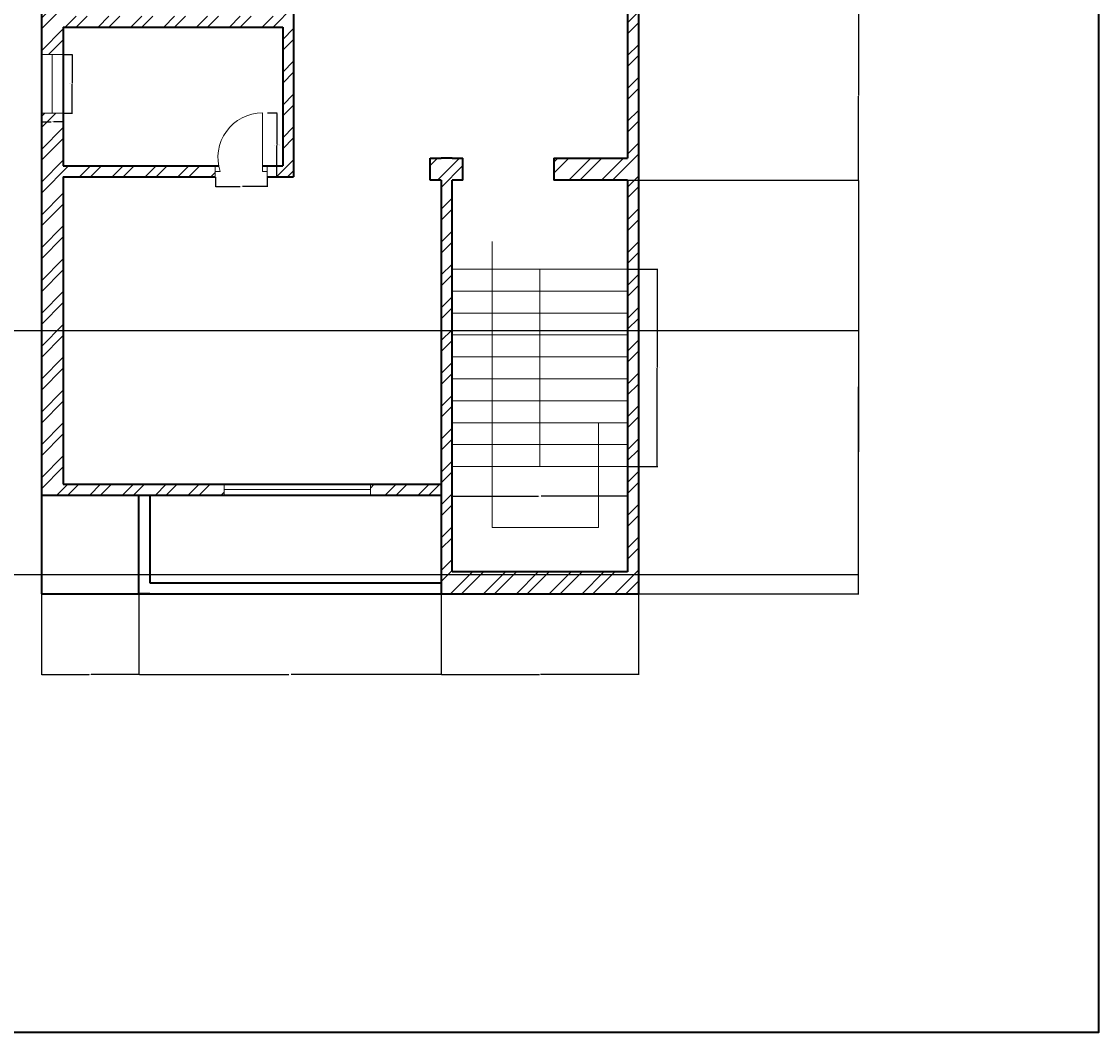
# Model space of a CAD drawing. Units: inches. Extents: x 1850 to 3445, y 1558 to 2756.
# Tile 11 of 13: x 3003 to 3445, y 1558 to 1972. Entities that reach past the tile are written whole.
import ezdxf

# ---------------------------------------------------------------- set-up
doc = ezdxf.new("R2010")
doc.units = ezdxf.units.IN
for name, color, linetype, lineweight in [('A-ANNO-DIMS', 2, 'Continuous', 18), ('A-ANNO-TTLB', 7, 'Continuous', 35), ('A-DOOR', 3, 'Continuous', 18), ('A-FLOR-STRS', 7, 'Continuous', 18), ('A-GLAZ', 4, 'Continuous', 18), ('A-WALL', 7, 'Continuous', 35), ('A-WALL-PATT', 252, 'Continuous', 13)]:
    doc.layers.add(name, color=color, linetype=linetype, lineweight=lineweight)
doc.styles.get("Standard").update_dxf_attribs({"font": 'arial.ttf'})
doc.dimstyles.get("Standard").update_dxf_attribs({"dimtxt": 0.18, "dimasz": 0.18, "dimexe": 0.18, "dimexo": 0.0625, "dimgap": 0.09, "dimtad": 0, "dimtih": 1, "dimtoh": 1, "dimdec": 4, "dimzin": 0, "dimdsep": 46, "dimtxsty": 'Standard', "dimcen": 0.09, "dimadec": 0, "dimazin": 0, "dimtfac": 1, "dimtdec": 4, "dimtofl": 0, "dimtmove": 0, "dimatfit": 3, "dimfxl": 1, "dimtolj": 1, "dimtzin": 0, "dimarcsym": 0})
pattern_1 = [(45, (660.551, 0), (-6.735192, 6.735192), []), (45, (665.041, 0), (-6.735192, 6.735192), [])]

# ---------------------------------------------------------------- blocks, each defined once
blk = doc.blocks.new('WIN-24-W9')
for p, q in [((9, 24), (0, 24)), ((0, 24), (4.5, 24)), ((4.5, 24), (4.5, 0)), ((9, 0), (0, 0)), ((4.5, 0), (9, 0))]:
    blk.add_line(p, q)
blk = doc.blocks.new('WIN-60-W4_5')
for p, q in [((0, 60), (4.5, 60)), ((4.5, 60), (2.25, 60)), ((2.25, 60), (2.25, 0)), ((2.25, 0), (0, 0)), ((0, 0), (4.5, 0))]:
    blk.add_line(p, q)
blk = doc.blocks.new('DOOR-BATH-LOWER-HALL')
for p, q in [((19.31, 2.25), (19.31, 26.25)), ((0, 4.5), (0, 0)), ((21.31, 4.5), (21.31, 0)), ((0, 0), (0, 2.25)), ((0, 2.25), (2, 2.25)), ((21.31, 2.25), (19.31, 2.25)), ((21.31, 0), (21.31, 2.25))]:
    blk.add_line(p, q)
blk.add_arc((19.31, 8.01), 18.24, 90, 198.4026)
blk = doc.blocks.new('STAIR-UPPER-FLIGHT')
for p, q in [((72, 81), (0, 81)), ((36, 0), (36, 81)), ((72, 72), (0, 72)), ((72, 63), (0, 63)), ((72, 54), (0, 54)), ((72, 45), (0, 45)), ((72, 36), (0, 36)), ((72, 27), (0, 27)), ((72, 18), (0, 18)), ((72, 9), (0, 9)), ((0, 0), (72, 0)), ((72, 0), (36, 0))]:
    blk.add_line(p, q)
blk = doc.blocks.new('*D40')
at = {"layer": 'A-ANNO-DIMS', "color": 0, "lineweight": -2, "transparency": 16777216}
for p, q in [((3020.67, 1958.91), (3024.39, 1958.91)), ((3024.21, 1958.73), (3024.21, 1947.1)), ((3024.21, 1935.09), (3024.21, 1946.73)), ((3020.67, 1934.91), (3024.39, 1934.91))]:
    blk.add_line(p, q, dxfattribs=at)
at = {"layer": 'A-ANNO-DIMS', "color": 0, "transparency": 16777216}
for points in [[(3024.18, 1958.73), (3024.24, 1958.73), (3024.21, 1958.91)], [(3024.18, 1935.09), (3024.24, 1935.09), (3024.21, 1934.91)]]:
    blk.add_solid(points, dxfattribs=at)
at = {"layer": 'Defpoints', "color": 0, "transparency": 16777216}
for p in [(3020.61, 1958.91), (3024.21, 1958.91), (3020.61, 1934.91)]:
    blk.add_point(p, dxfattribs=at)
at = {"layer": 'A-ANNO-DIMS', "color": 0, "transparency": 16777216, "insert": (3024.21, 1946.91), "char_height": 0.18, "attachment_point": 5}
blk.add_mtext('\\A1;WINDOW 24 TYP.', dxfattribs=at)
blk = doc.blocks.new('*D41')
at = {"layer": 'A-ANNO-DIMS', "color": 0, "lineweight": -2, "transparency": 16777216}
for p, q in [((3011.61, 1934.85), (3011.61, 1931.13)), ((3011.79, 1931.31), (3015.65, 1931.31)), ((3020.43, 1931.31), (3016.56, 1931.31)), ((3020.61, 1934.85), (3020.61, 1931.13))]:
    blk.add_line(p, q, dxfattribs=at)
at = {"layer": 'A-ANNO-DIMS', "color": 0, "transparency": 16777216}
for points in [[(3011.79, 1931.34), (3011.79, 1931.28), (3011.61, 1931.31)], [(3020.43, 1931.34), (3020.43, 1931.28), (3020.61, 1931.31)]]:
    blk.add_solid(points, dxfattribs=at)
at = {"layer": 'Defpoints', "color": 0, "transparency": 16777216}
for p in [(3011.61, 1934.91), (3020.61, 1934.91), (3020.61, 1931.31)]:
    blk.add_point(p, dxfattribs=at)
at = {"layer": 'A-ANNO-DIMS', "color": 0, "transparency": 16777216, "insert": (3016.11, 1931.31), "char_height": 0.18, "attachment_point": 5}
blk.add_mtext('\\A1;9 TYP.', dxfattribs=at)
blk = doc.blocks.new('*D66')
at = {"layer": 'A-ANNO-DIMS', "color": 0, "lineweight": -2, "transparency": 16777216}
for p, q in [((3104.35, 1934.93), (3108.4, 1934.93)), ((3108.22, 1934.75), (3108.22, 1921.99)), ((3108.22, 1908.86), (3108.22, 1921.63)), ((3104.35, 1908.68), (3108.4, 1908.68))]:
    blk.add_line(p, q, dxfattribs=at)
at = {"layer": 'A-ANNO-DIMS', "color": 0, "transparency": 16777216}
for points in [[(3108.19, 1934.75), (3108.25, 1934.75), (3108.22, 1934.93)], [(3108.19, 1908.86), (3108.25, 1908.86), (3108.22, 1908.68)]]:
    blk.add_solid(points, dxfattribs=at)
at = {"layer": 'Defpoints', "color": 0, "transparency": 16777216}
for p in [(3104.28, 1934.93), (3108.22, 1934.93), (3104.28, 1908.68)]:
    blk.add_point(p, dxfattribs=at)
at = {"layer": 'A-ANNO-DIMS', "color": 0, "transparency": 16777216, "insert": (3108.22, 1921.81), "char_height": 0.18, "attachment_point": 5}
blk.add_mtext('\\A1;BATH DOOR 26 TYP.', dxfattribs=at)
blk = doc.blocks.new('*D67')
at = {"layer": 'A-ANNO-DIMS', "color": 0, "lineweight": -2, "transparency": 16777216}
for p, q in [((3082.98, 1908.62), (3082.98, 1904.57)), ((3104.28, 1908.62), (3104.28, 1904.57)), ((3083.16, 1904.75), (3093.1, 1904.75)), ((3104.1, 1904.75), (3094.16, 1904.75))]:
    blk.add_line(p, q, dxfattribs=at)
at = {"layer": 'A-ANNO-DIMS', "color": 0, "transparency": 16777216}
for points in [[(3083.16, 1904.78), (3083.16, 1904.72), (3082.98, 1904.75)], [(3104.1, 1904.78), (3104.1, 1904.72), (3104.28, 1904.75)]]:
    blk.add_solid(points, dxfattribs=at)
at = {"layer": 'Defpoints', "color": 0, "transparency": 16777216}
for p in [(3082.98, 1908.68), (3104.28, 1908.68), (3104.28, 1904.75)]:
    blk.add_point(p, dxfattribs=at)
at = {"layer": 'A-ANNO-DIMS', "color": 0, "transparency": 16777216, "insert": (3093.63, 1904.75), "char_height": 0.18, "attachment_point": 5}
blk.add_mtext('\\A1;21 TYP.', dxfattribs=at)
blk = doc.blocks.new('*D70')
at = {"layer": 'A-ANNO-DIMS', "color": 0, "lineweight": -2, "transparency": 16777216}
for p, q in [((3252.17, 1870.88), (3264.44, 1870.88)), ((3264.26, 1870.7), (3264.26, 1830.56)), ((3264.26, 1790.06), (3264.26, 1830.2)), ((3252.17, 1789.88), (3264.44, 1789.88))]:
    blk.add_line(p, q, dxfattribs=at)
at = {"layer": 'A-ANNO-DIMS', "color": 0, "transparency": 16777216}
for points in [[(3264.23, 1870.7), (3264.29, 1870.7), (3264.26, 1870.88)], [(3264.23, 1790.06), (3264.29, 1790.06), (3264.26, 1789.88)]]:
    blk.add_solid(points, dxfattribs=at)
at = {"layer": 'Defpoints', "color": 0, "transparency": 16777216}
for p in [(3252.11, 1870.88), (3264.26, 1870.88), (3252.11, 1789.88)]:
    blk.add_point(p, dxfattribs=at)
at = {"layer": 'A-ANNO-DIMS', "color": 0, "transparency": 16777216, "insert": (3264.26, 1830.38), "char_height": 0.18, "attachment_point": 5}
blk.add_mtext('\\A1;STAIR FLIGHT 81 TYP.', dxfattribs=at)
blk = doc.blocks.new('*D71')
at = {"layer": 'A-ANNO-DIMS', "color": 0, "lineweight": -2, "transparency": 16777216}
for p, q in [((3180.11, 1789.82), (3180.11, 1777.55)), ((3252.11, 1789.82), (3252.11, 1777.55)), ((3180.29, 1777.73), (3215.58, 1777.73)), ((3251.93, 1777.73), (3216.63, 1777.73))]:
    blk.add_line(p, q, dxfattribs=at)
at = {"layer": 'A-ANNO-DIMS', "color": 0, "transparency": 16777216}
for points in [[(3180.29, 1777.76), (3180.29, 1777.7), (3180.11, 1777.73)], [(3251.93, 1777.76), (3251.93, 1777.7), (3252.11, 1777.73)]]:
    blk.add_solid(points, dxfattribs=at)
at = {"layer": 'Defpoints', "color": 0, "transparency": 16777216}
for p in [(3180.11, 1789.88), (3252.11, 1789.88), (3252.11, 1777.73)]:
    blk.add_point(p, dxfattribs=at)
at = {"layer": 'A-ANNO-DIMS', "color": 0, "transparency": 16777216, "insert": (3216.11, 1777.73), "char_height": 0.18, "attachment_point": 5}
blk.add_mtext('\\A1;72 TYP.', dxfattribs=at)
blk = doc.blocks.new('*D94')
at = {"layer": 'A-ANNO-DIMS', "color": 0, "lineweight": -2, "transparency": 16777216}
for p, q in [((3011.61, 1737.62), (3011.61, 1704.45)), ((3051.65, 1737.62), (3051.65, 1704.45)), ((3011.79, 1704.63), (3031.16, 1704.63)), ((3051.47, 1704.63), (3032.1, 1704.63))]:
    blk.add_line(p, q, dxfattribs=at)
at = {"layer": 'A-ANNO-DIMS', "color": 0, "transparency": 16777216}
for points in [[(3011.79, 1704.66), (3011.79, 1704.6), (3011.61, 1704.63)], [(3051.47, 1704.66), (3051.47, 1704.6), (3051.65, 1704.63)]]:
    blk.add_solid(points, dxfattribs=at)
at = {"layer": 'Defpoints', "color": 0, "transparency": 16777216}
for p in [(3011.61, 1737.68), (3051.65, 1737.68), (3051.65, 1704.63)]:
    blk.add_point(p, dxfattribs=at)
at = {"layer": 'A-ANNO-DIMS', "color": 0, "transparency": 16777216, "insert": (3031.63, 1704.63), "char_height": 0.18, "attachment_point": 5}
blk.add_mtext('\\A1;40.046', dxfattribs=at)
blk = doc.blocks.new('*D95')
at = {"layer": 'A-ANNO-DIMS', "color": 0, "lineweight": -2, "transparency": 16777216}
for p, q in [((3051.65, 1737.62), (3051.65, 1704.45)), ((3175.61, 1737.62), (3175.61, 1704.45)), ((3051.83, 1704.63), (3113.17, 1704.63)), ((3175.43, 1704.63), (3114.08, 1704.63))]:
    blk.add_line(p, q, dxfattribs=at)
at = {"layer": 'A-ANNO-DIMS', "color": 0, "transparency": 16777216}
for points in [[(3051.83, 1704.66), (3051.83, 1704.6), (3051.65, 1704.63)], [(3175.43, 1704.66), (3175.43, 1704.6), (3175.61, 1704.63)]]:
    blk.add_solid(points, dxfattribs=at)
at = {"layer": 'Defpoints', "color": 0, "transparency": 16777216}
for p in [(3051.65, 1737.68), (3175.61, 1737.68), (3175.61, 1704.63)]:
    blk.add_point(p, dxfattribs=at)
at = {"layer": 'A-ANNO-DIMS', "color": 0, "transparency": 16777216, "insert": (3113.63, 1704.63), "char_height": 0.18, "attachment_point": 5}
blk.add_mtext('\\A1;123.95', dxfattribs=at)
blk = doc.blocks.new('*D96')
at = {"layer": 'A-ANNO-DIMS', "color": 0, "lineweight": -2, "transparency": 16777216}
for p, q in [((3175.61, 1737.62), (3175.61, 1704.45)), ((3256.61, 1737.62), (3256.61, 1704.45)), ((3175.79, 1704.63), (3215.9, 1704.63)), ((3256.43, 1704.63), (3216.31, 1704.63))]:
    blk.add_line(p, q, dxfattribs=at)
at = {"layer": 'A-ANNO-DIMS', "color": 0, "transparency": 16777216}
for points in [[(3175.79, 1704.66), (3175.79, 1704.6), (3175.61, 1704.63)], [(3256.43, 1704.66), (3256.43, 1704.6), (3256.61, 1704.63)]]:
    blk.add_solid(points, dxfattribs=at)
at = {"layer": 'Defpoints', "color": 0, "transparency": 16777216}
for p in [(3175.61, 1737.68), (3256.61, 1737.68), (3256.61, 1704.63)]:
    blk.add_point(p, dxfattribs=at)
at = {"layer": 'A-ANNO-DIMS', "color": 0, "transparency": 16777216, "insert": (3216.11, 1704.63), "char_height": 0.18, "attachment_point": 5}
blk.add_mtext('\\A1;81', dxfattribs=at)
blk = doc.blocks.new('*D102')
at = {"layer": 'A-ANNO-DIMS', "color": 0, "lineweight": -2, "transparency": 16777216}
for p, q in [((2941.38, 1845.68), (3346.97, 1845.68)), ((3346.79, 1845.5), (3346.79, 1795.87)), ((3346.79, 1745.86), (3346.79, 1795.5)), ((2945.88, 1745.68), (3346.97, 1745.68))]:
    blk.add_line(p, q, dxfattribs=at)
at = {"layer": 'A-ANNO-DIMS', "color": 0, "transparency": 16777216}
for points in [[(3346.76, 1845.5), (3346.82, 1845.5), (3346.79, 1845.68)], [(3346.76, 1745.86), (3346.82, 1745.86), (3346.79, 1745.68)]]:
    blk.add_solid(points, dxfattribs=at)
at = {"layer": 'Defpoints', "color": 0, "transparency": 16777216}
for p in [(2941.32, 1845.68), (3346.79, 1845.68), (2945.82, 1745.68)]:
    blk.add_point(p, dxfattribs=at)
at = {"layer": 'A-ANNO-DIMS', "color": 0, "transparency": 16777216, "insert": (3346.79, 1795.68), "char_height": 0.18, "attachment_point": 5}
blk.add_mtext('\\A1;100', dxfattribs=at)
blk = doc.blocks.new('*D103')
at = {"layer": 'A-ANNO-DIMS', "color": 0, "lineweight": -2, "transparency": 16777216}
for p, q in [((3252.17, 1907.39), (3346.97, 1907.39)), ((3346.79, 1907.21), (3346.79, 1822.72)), ((3346.79, 1737.86), (3346.79, 1822.36)), ((3256.67, 1737.68), (3346.97, 1737.68))]:
    blk.add_line(p, q, dxfattribs=at)
at = {"layer": 'A-ANNO-DIMS', "color": 0, "transparency": 16777216}
for points in [[(3346.76, 1907.21), (3346.82, 1907.21), (3346.79, 1907.39)], [(3346.76, 1737.86), (3346.82, 1737.86), (3346.79, 1737.68)]]:
    blk.add_solid(points, dxfattribs=at)
at = {"layer": 'Defpoints', "color": 0, "transparency": 16777216}
for p in [(3252.11, 1907.39), (3346.79, 1907.39), (3256.61, 1737.68)]:
    blk.add_point(p, dxfattribs=at)
at = {"layer": 'A-ANNO-DIMS', "color": 0, "transparency": 16777216, "insert": (3346.79, 1822.54), "char_height": 0.18, "attachment_point": 5}
blk.add_mtext('\\A1;169.7', dxfattribs=at)
blk = doc.blocks.new('*D104')
at = {"layer": 'A-ANNO-DIMS', "color": 0, "lineweight": -2, "transparency": 16777216}
for p, q in [((3256.67, 1976.5), (3346.97, 1976.5)), ((3346.79, 1976.32), (3346.79, 1942.13)), ((3346.79, 1907.57), (3346.79, 1941.76)), ((3252.17, 1907.39), (3346.97, 1907.39))]:
    blk.add_line(p, q, dxfattribs=at)
at = {"layer": 'A-ANNO-DIMS', "color": 0, "transparency": 16777216}
for points in [[(3346.76, 1976.32), (3346.82, 1976.32), (3346.79, 1976.5)], [(3346.76, 1907.57), (3346.82, 1907.57), (3346.79, 1907.39)]]:
    blk.add_solid(points, dxfattribs=at)
at = {"layer": 'Defpoints', "color": 0, "transparency": 16777216}
for p in [(3256.61, 1976.5), (3346.79, 1976.5), (3252.11, 1907.39)]:
    blk.add_point(p, dxfattribs=at)
at = {"layer": 'A-ANNO-DIMS', "color": 0, "transparency": 16777216, "insert": (3346.79, 1941.94), "char_height": 0.18, "attachment_point": 5}
blk.add_mtext('\\A1;69.1', dxfattribs=at)

msp = doc.modelspace()

# ---------------------------------------------------------------- hatches: boundary and pattern name
at = {"layer": 'A-WALL-PATT'}
h = msp.add_hatch(dxfattribs=at)
h.set_pattern_fill('ANSI32', color=256)
h.set_pattern_definition(pattern_1)
h.paths.add_polyline_path([(3180.1061, 1907.3936), (3184.5492, 1907.3936), (3184.5492, 1916.3936), (3180.1061, 1916.3936), (3175.6061, 1916.3936), (3171.1061, 1916.3936), (3171.1061, 1907.3936), (3175.6061, 1907.3936), (3175.6061, 1742.1843), (3175.6061, 1737.6843), (3256.6061, 1737.6843), (3256.6061, 1976.4962), (3252.1061, 1976.4962), (3252.1061, 1916.3936), (3221.8172, 1916.3936), (3221.8172, 1907.3936), (3252.1061, 1907.3936), (3252.1061, 1746.6843), (3180.1061, 1746.6843)])
h.paths.add_polyline_path([(2737.1986, 2211.6843), (2737.1986, 2216.1843), (2700.822, 2216.1843), (2700.822, 2175.83), (2705.322, 2175.83), (2709.822, 2175.83), (2709.822, 2207.1843), (2737.1986, 2207.1843)])
h.paths.add_polyline_path([(2872.322, 2216.1843), (2797.1986, 2216.1843), (2797.1986, 2207.1843), (2872.322, 2207.1843)])
h.paths.add_polyline_path([(2945.822, 2154.1843), (2911.1674, 2154.1843), (2911.1674, 2149.6843), (2941.322, 2149.6843), (2941.322, 2075.1843), (2896.9138, 2075.1843), (2896.9138, 2070.6843), (2945.822, 2070.6843)])
h.paths.add_polyline_path([(2888.8991, 2154.1843), (2867.822, 2154.1843), (2867.822, 2075.1843), (2862.5325, 2075.1843), (2862.5325, 2070.6843), (2876.0169, 2070.6843), (2876.0169, 2072.9343), (2876.0169, 2075.1843), (2872.322, 2075.1843), (2872.322, 2149.6843), (2888.8991, 2149.6843)])
h.paths.add_polyline_path([(2709.822, 2115.83), (2700.822, 2115.83), (2700.822, 2042.8465), (2709.822, 2042.8465), (2709.822, 2070.6843), (2829.1562, 2070.6843), (2829.1562, 2072.9343), (2829.1562, 2075.1843), (2709.822, 2075.1843)])
h.paths.add_polyline_path([(2709.822, 1982.8465), (2700.822, 1982.8465), (2700.822, 1910.2175), (2721.4986, 1910.2175), (2721.4986, 1914.7175), (2721.4986, 1919.2175), (2709.822, 1919.2175)])
h.paths.add_polyline_path([(2793.0443, 1919.2175), (2769.4986, 1919.2175), (2769.4986, 1910.2175), (2793.0443, 1910.2175), (2793.0443, 1914.6749)])
h.paths.add_polyline_path([(2839.322, 1938.6843), (2830.322, 1938.6843), (2830.322, 1919.2175), (2824.2376, 1919.2175), (2824.2376, 1910.2175), (2830.322, 1910.2175), (2830.322, 1854.6843), (2830.322, 1845.6843), (2856.6792, 1845.6843), (2856.6792, 1850.1843), (2856.6792, 1854.6843), (2839.322, 1854.6843)])
h.paths.add_polyline_path([(2709.822, 1910.2175), (2700.822, 1910.2175), (2700.822, 1745.6843), (2709.822, 1745.6843)])
h.paths.add_polyline_path([(2807.4367, 1766.7204), (2819.64, 1766.7204), (2819.64, 1777.0239), (2807.4367, 1777.0239)], flags=9)
h.paths.add_polyline_path([(2844.0169, 1798.4016), (2887.2843, 1798.4016), (2887.2843, 1817.0589), (2844.0169, 1817.0589)], flags=9)
h.paths.add_polyline_path([(2731.4135, 1867.537), (2770.5302, 1867.537), (2770.5302, 1886.1943), (2731.4135, 1886.1943)], flags=9)
h = msp.add_hatch(dxfattribs=at)
h.set_pattern_fill('ANSI32', color=256)
h.set_pattern_definition(pattern_1)
h.paths.add_polyline_path([(3064.1082, 2211.6843), (3064.1082, 2216.1843), (3011.6061, 2216.1843), (3011.6061, 2169.0079), (3020.6061, 2169.0079), (3020.6061, 2207.1843), (3064.1082, 2207.1843)])
h.paths.add_polyline_path([(3183.1061, 2216.1843), (3124.1082, 2216.1843), (3124.1082, 2207.1843), (3183.1061, 2207.1843)])
h.paths.add_polyline_path([(3256.6061, 2154.1843), (3223.2152, 2154.1843), (3223.2152, 2149.6843), (3252.1061, 2149.6843), (3252.1061, 2075.1843), (3183.1061, 2075.1843), (3183.1061, 2079.8699), (3178.6061, 2079.8699), (3178.6061, 2075.1843), (3172.4917, 2075.1843), (3172.4917, 2070.6843), (3252.1061, 2070.6843), (3252.1061, 2036.4962), (3256.6061, 2036.4962)])
h.paths.add_polyline_path([(3199.2152, 2154.1843), (3183.1061, 2154.1843), (3178.6061, 2154.1843), (3178.6061, 2102.7998), (3183.1061, 2102.7998), (3183.1061, 2149.6843), (3199.2152, 2149.6843)], flags=17)
h.paths.add_polyline_path([(3138.4194, 2072.9343), (3138.4194, 2075.1843), (3020.6061, 2075.1843), (3020.6061, 2109.0079), (3016.1061, 2109.0079), (3011.6061, 2109.0079), (3011.6061, 2043.8694), (3016.1061, 2043.8694), (3020.6061, 2043.8694), (3020.6061, 2070.6843), (3110.6061, 2070.6843), (3110.6061, 2045.0271), (3115.1061, 2045.0271), (3115.1061, 2070.6843), (3138.4194, 2070.6843)])
h.paths.add_polyline_path([(3020.6061, 2007.8694), (3011.6061, 2007.8694), (3011.6061, 1958.9131), (3016.1061, 1958.9131), (3020.6061, 1958.9131), (3020.6061, 1970.1843), (3110.6061, 1970.1843), (3110.6061, 1913.1843), (3104.2838, 1913.1843), (3104.2838, 1908.6843), (3115.1061, 1908.6843), (3115.1061, 1999.4184), (3110.6061, 1999.4184), (3110.6061, 1974.6843), (3020.6061, 1974.6843)])
h.paths.add_polyline_path([(3020.6061, 1908.6843), (3082.9753, 1908.6843), (3082.9753, 1910.9343), (3082.9753, 1913.1843), (3020.6061, 1913.1843), (3020.6061, 1934.9131), (3011.6061, 1934.9131), (3011.6061, 1778.1843), (3086.5835, 1778.1843), (3086.5835, 1780.4343), (3086.5835, 1782.6843), (3020.6061, 1782.6843)])
h.paths.add_polyline_path([(3175.6061, 1782.6843), (3146.5835, 1782.6843), (3146.5835, 1778.1843), (3175.6061, 1778.1843)])

# ---------------------------------------------------------------- linework, layer by layer
at = {"layer": 'A-ANNO-TTLB'}
msp.add_lwpolyline([(1850.1793, 2756.3177), (3445.2682, 2756.3177), (3445.2682, 1557.7728), (1850.1793, 1557.7728)], close=True, dxfattribs=at)
at = {"layer": 'A-FLOR-STRS'}
for p, q in [((3196.585, 1882.1893), (3196.585, 1764.8415)), ((3240.1998, 1764.8415), (3240.1998, 1807.8818)), ((3196.585, 1764.8415), (3240.1998, 1764.8415))]:
    msp.add_line(p, q, dxfattribs=at)
at = {"layer": 'A-WALL'}
for p, q in [((3011.6061, 2216.1843), (3011.6061, 1737.6843)), ((3256.6061, 2216.1843), (3256.6061, 1737.6843)), ((3252.1061, 2070.6843), (3252.1061, 1916.3936)), ((3115.1061, 1999.4184), (3115.1061, 1908.6843)), ((3020.6061, 1970.1843), (3110.6061, 1970.1843)), ((3020.6061, 1970.1843), (3020.6061, 1913.1843)), ((3110.6061, 1970.1843), (3110.6061, 1913.1843)), ((3020.6061, 1913.1843), (3084.3831, 1913.1843)), ((3102.2838, 1913.1843), (3110.6061, 1913.1843)), ((3171.1061, 1907.3936), (3171.1061, 1916.3936)), ((3171.1061, 1916.3936), (3175.6061, 1916.3936)), ((3180.1061, 1916.3936), (3175.6061, 1916.3936)), ((3180.1061, 1916.3936), (3184.5492, 1916.3936)), ((3184.5492, 1907.3936), (3184.5492, 1916.3936)), ((3221.8172, 1916.3936), (3252.1061, 1916.3936)), ((3221.8172, 1916.3936), (3221.8172, 1907.3936)), ((3020.6061, 1908.6843), (3082.9753, 1908.6843)), ((3020.6061, 1908.6843), (3020.6061, 1782.6843)), ((3104.2838, 1908.6843), (3115.1061, 1908.6843)), ((3175.6061, 1907.3936), (3171.1061, 1907.3936)), ((3175.6061, 1907.3936), (3175.6061, 1742.1843)), ((3180.1061, 1746.6843), (3180.1061, 1907.3936)), ((3184.5492, 1907.3936), (3180.1061, 1907.3936)), ((3252.1061, 1907.3936), (3221.8172, 1907.3936)), ((3252.1061, 1907.3936), (3252.1061, 1746.6843)), ((3020.6061, 1782.6843), (3175.6061, 1782.6843)), ((3011.6061, 1778.1843), (3175.6061, 1778.1843)), ((3051.652, 1737.6843), (3051.652, 1778.1843)), ((3056.152, 1778.1843), (3056.152, 1742.1843)), ((3252.1061, 1746.6843), (3180.1061, 1746.6843)), ((3056.152, 1742.1843), (3175.6061, 1742.1843)), ((3175.6061, 1742.1843), (3175.6061, 1737.6843)), ((3011.6061, 1737.6843), (3256.6061, 1737.6843)), ((3056.152, 1737.6843), (3051.652, 1737.6843))]:
    msp.add_line(p, q, dxfattribs=at)

# ---------------------------------------------------------------- block references
at = {"layer": 'A-DOOR'}
msp.add_blockref('DOOR-BATH-LOWER-HALL', (3082.9755, 1908.684), dxfattribs=at)
at = {"layer": 'A-FLOR-STRS'}
msp.add_blockref('STAIR-UPPER-FLIGHT', (3180.1065, 1789.882), dxfattribs=at)
at = {"layer": 'A-GLAZ'}
msp.add_blockref('WIN-24-W9', (3011.6065, 1934.913), dxfattribs=at)
at = {"layer": 'A-GLAZ', "extrusion": (0, 0, -1), "zscale": -1, "rotation": 90}
msp.add_blockref('WIN-60-W4_5', (-3086.5835, 1778.1838), dxfattribs=at)

# ---------------------------------------------------------------- dimensions: what is measured, and where the dimension line sits
at = {"layer": 'A-ANNO-DIMS'}
for base, p1, p2, override, picture, middle in [((3346.7887, 1976.4962), (3252.1061, 1907.3936), (3256.6061, 1976.4962), {"dimdec": 1, "dimlfac": 1, "dimrnd": 0, "dimzin": 0, "dimdsep": 46, "dimlunit": 2}, '*D104', (3346.7887, 1941.9449)), ((3346.7887, 1907.3936), (3256.6061, 1737.6843), (3252.1061, 1907.3936), {"dimdec": 1, "dimlfac": 1, "dimrnd": 0, "dimzin": 0, "dimdsep": 46, "dimlunit": 2}, '*D103', (3346.7887, 1822.5389)), ((3346.7887, 1845.6843), (2945.822, 1745.6843), (2941.322, 1845.6843), {"dimdec": 0, "dimlfac": 1, "dimrnd": 0, "dimzin": 0, "dimdsep": 46, "dimlunit": 2}, '*D102', (3346.7887, 1795.6843))]:
    dim = msp.add_linear_dim(base=base, p1=p1, p2=p2, angle=90, dimstyle='Standard', override=override, dxfattribs=at)
    dim.commit()
    dim.dimension.update_dxf_attribs({"geometry": picture, "text_midpoint": middle})
for base, p1, p2, text, picture, middle in [((3024.2061, 1958.9131), (3020.6061, 1934.9131), (3020.6061, 1958.9131), 'WINDOW <> TYP.', '*D40', (3024.2061, 1946.9131)), ((3108.2213, 1934.9343), (3104.2838, 1908.6843), (3104.2838, 1934.9343), 'BATH DOOR <> TYP.', '*D66', (3108.2213, 1921.8093)), ((3264.2561, 1870.8818), (3252.1061, 1789.8818), (3252.1061, 1870.8818), 'STAIR FLIGHT <> TYP.', '*D70', (3264.2561, 1830.3818))]:
    dim = msp.add_linear_dim(base=base, p1=p1, p2=p2, angle=90, text=text, dimstyle='Standard', override={"dimdec": 0, "dimlfac": 1, "dimrnd": 0, "dimzin": 0, "dimdsep": 46, "dimlunit": 2}, dxfattribs=at)
    dim.commit()
    dim.dimension.update_dxf_attribs({"geometry": picture, "text_midpoint": middle})
for base, p1, p2, picture, middle in [((3020.6061, 1931.3131), (3011.6061, 1934.9131), (3020.6061, 1934.9131), '*D41', (3016.1061, 1931.3131)), ((3104.2838, 1904.7468), (3082.9753, 1908.6843), (3104.2838, 1908.6843), '*D67', (3093.6295, 1904.7468)), ((3252.1061, 1777.7318), (3180.1061, 1789.8818), (3252.1061, 1789.8818), '*D71', (3216.1061, 1777.7318))]:
    dim = msp.add_linear_dim(base=base, p1=p1, p2=p2, text='<> TYP.', dimstyle='Standard', override={"dimdec": 0, "dimlfac": 1, "dimrnd": 0, "dimzin": 0, "dimdsep": 46, "dimlunit": 2}, dxfattribs=at)
    dim.commit()
    dim.dimension.update_dxf_attribs({"geometry": picture, "text_midpoint": middle})
for base, p1, p2, override, picture, middle in [((3051.652, 1704.6343), (3011.6061, 1737.6843), (3051.652, 1737.6843), {"dimdec": 3, "dimlfac": 1, "dimrnd": 0, "dimzin": 0, "dimdsep": 46, "dimlunit": 2}, '*D94', (3031.6291, 1704.6343)), ((3175.6061, 1704.6343), (3051.652, 1737.6843), (3175.6061, 1737.6843), {"dimdec": 2, "dimlfac": 1, "dimrnd": 0, "dimzin": 0, "dimdsep": 46, "dimlunit": 2}, '*D95', (3113.6291, 1704.6343)), ((3256.6061, 1704.6343), (3175.6061, 1737.6843), (3256.6061, 1737.6843), {"dimdec": 0, "dimlfac": 1, "dimrnd": 0, "dimzin": 0, "dimdsep": 46, "dimlunit": 2}, '*D96', (3216.1061, 1704.6343))]:
    dim = msp.add_linear_dim(base=base, p1=p1, p2=p2, dimstyle='Standard', override=override, dxfattribs=at)
    dim.commit()
    dim.dimension.update_dxf_attribs({"geometry": picture, "text_midpoint": middle})

doc.saveas('drawing.dxf')
